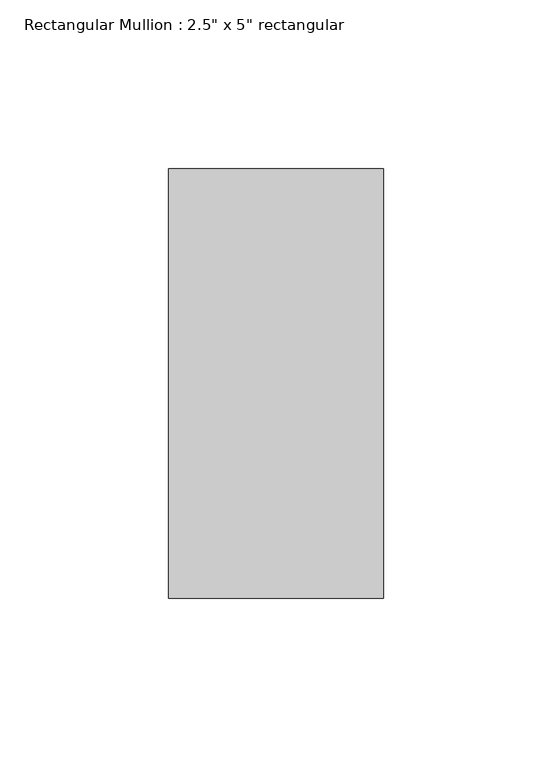
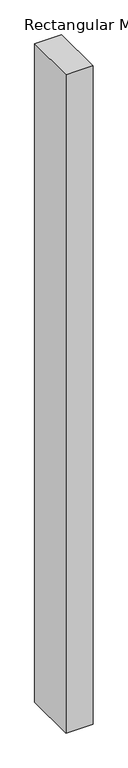
"""IFC4 building model written with IfcOpenShell, lengths in millimetres: member geometry."""

from ifc_helpers import new_model, si_unit, frame, origin, place, context, project, spatial, polyline, outline, extrude, source, transform, mapped, element, save


def member_1e79e512(model_context):
    return source(origin(), model_context, "Body", "SweptSolid", [
        extrude(outline(polyline([(0.0, 63.5), (0.0, -63.5), (-63.5, -63.5), (-63.5, 63.5), (0.0, 63.5)])), frame((0.0, 0.0, -1633.7500384), z_axis=(0.0, 0.0, 1.0), x_axis=(1.0, 0.0, 0.0)), (0.0, 0.0, 1.0), 1633.7500384),
    ])


if __name__ == "__main__":
    model = new_model("IFC4")
    model_context = context("Model", 3, world=origin())
    ifc_project = project(units=[si_unit("LENGTHUNIT", "METRE", prefix="MILLI")], contexts=[model_context])
    site = spatial("IfcSite", under=ifc_project)
    building = spatial("IfcBuilding", under=site)
    placement = place(None, origin())
    member_shape = member_1e79e512(model_context)
    element("IfcMember", 1, ObjectType="Rectangular Mullion : 2.5\" x 5\" rectangular", at=placement, inside=building, context=model_context, shape_type="MappedRepresentation", body=[
        mapped(member_shape, transform((0.0, 0.0, 0.0), x_axis=(1.0, 0.0, 0.0), y_axis=(0.0, 1.0, 0.0), z_axis=(0.0, 0.0, 1.0))),
    ])
    save(model, "model.ifc")

# Revit data of these elements
# Type "Rectangular Mullion : 2.5\" x 5\" rectangular"
#   built-in parameter 1007304 = 0.416667 (stored number, unit not read)
#   built-in parameter 1007301 = 0.104167 (stored number, unit not read)
#   built-in parameter 1007300 = 0.104167 (stored number, unit not read)
# Element 1 (IfcMember, "Rectangular Mullion : 2.5\" x 5\" rectangular")
#   Materials on its faces: "Aluminum"
# Materials
#   "Aluminum": class "Metal", colour RGB 247 247 247, transparency 0, Description = "Aluminum 6061", Cost = 0
